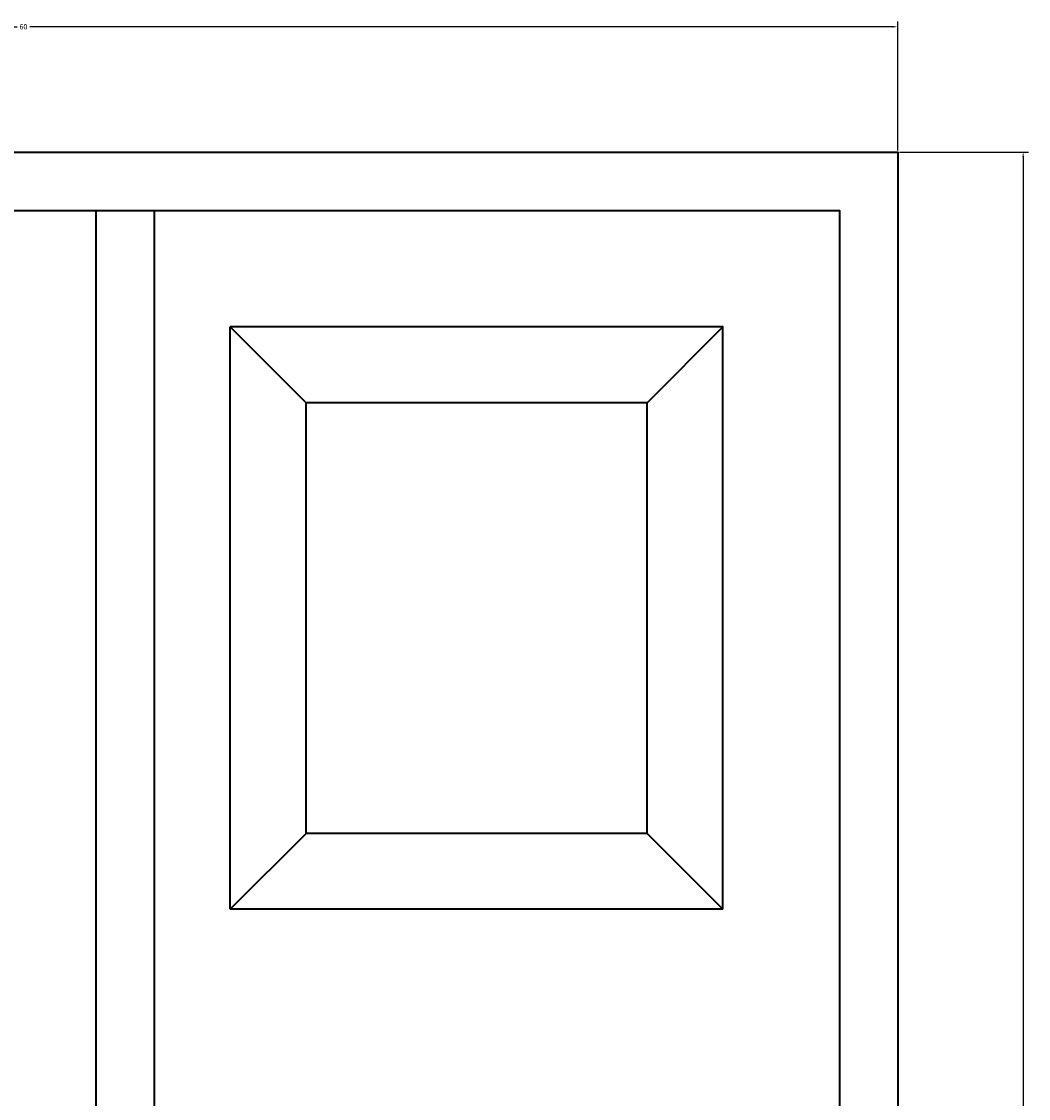
# Model space of a CAD drawing. Units: inches. Extents: x 3137 to 3299, y 1994 to 2089.
# Tile 14 of 14: x 3264 to 3299, y 2052 to 2089. Entities that reach past the tile are written whole.
import ezdxf

# ---------------------------------------------------------------- set-up
doc = ezdxf.new("R2010")
doc.units = ezdxf.units.IN
doc.header["$MEASUREMENT"] = 0
doc.layers.add('A-ANNO-DIMS', color=2, linetype='Continuous', lineweight=18)
doc.layers.add('A-DOOR', color=4, linetype='Continuous', lineweight=35)
doc.styles.get("Standard").update_dxf_attribs({"font": 'arial.ttf'})
doc.dimstyles.get("Standard").update_dxf_attribs({"dimtxt": 0.18, "dimasz": 0.18, "dimexe": 0.18, "dimexo": 0.0625, "dimgap": 0.09, "dimtad": 0, "dimtih": 1, "dimtoh": 1, "dimdec": 4, "dimzin": 0, "dimdsep": 46, "dimtxsty": 'Standard', "dimcen": 0.09, "dimadec": 0, "dimazin": 0, "dimtfac": 1, "dimtdec": 4, "dimtofl": 0, "dimtmove": 0, "dimatfit": 3, "dimfxl": 1, "dimtolj": 1, "dimtzin": 0, "dimarcsym": 0})

# ---------------------------------------------------------------- blocks, each defined once
blk = doc.blocks.new('DOOR-PANEL-RAISED-TOP')
for p, q in [((0, 19.99), (2.6, 17.39)), ((14.3, 17.39), (16.9, 19.99)), ((16.9, 0), (16.9, 19.99)), ((14.3, 2.6), (14.3, 17.39)), ((2.6, 2.6), (0, 0)), ((2.6, 2.6), (14.3, 2.6)), ((14.3, 2.6), (16.9, 0)), ((0, 0), (16.9, 0))]:
    blk.add_line(p, q)
for points in [[(0, 0), (0, 19.99), (16.9, 19.99)], [(2.6, 2.6), (2.6, 17.39), (14.3, 17.39)]]:
    blk.add_lwpolyline(points)
blk = doc.blocks.new('*D74')
at = {"layer": 'A-ANNO-DIMS', "color": 0, "lineweight": -2, "transparency": 16777216}
for p, q in [((3234.504, 2084.238), (3234.504, 2088.661)), ((3294.504, 2084.238), (3294.504, 2088.661)), ((3234.684, 2088.481), (3264.285, 2088.481)), ((3294.324, 2088.481), (3264.723, 2088.481))]:
    blk.add_line(p, q, dxfattribs=at)
at = {"layer": 'A-ANNO-DIMS', "color": 0, "transparency": 16777216}
for points in [[(3234.684, 2088.511), (3234.684, 2088.451), (3234.504, 2088.481)], [(3294.324, 2088.511), (3294.324, 2088.451), (3294.504, 2088.481)]]:
    blk.add_solid(points, dxfattribs=at)
at = {"layer": 'Defpoints', "color": 0, "transparency": 16777216}
for p in [(3294.504, 2088.481), (3234.504, 2084.176), (3294.504, 2084.176)]:
    blk.add_point(p, dxfattribs=at)
at = {"layer": 'A-ANNO-DIMS', "color": 0, "transparency": 16777216, "insert": (3264.504, 2088.481), "char_height": 0.18, "attachment_point": 5}
blk.add_mtext('\\A1;60', dxfattribs=at)
blk = doc.blocks.new('*D75')
at = {"layer": 'A-ANNO-DIMS', "color": 0, "lineweight": -2, "transparency": 16777216}
for p, q in [((3294.566, 2084.176), (3298.989, 2084.176)), ((3298.809, 2083.996), (3298.809, 2042.358)), ((3298.809, 2000.356), (3298.809, 2041.994)), ((3294.566, 2000.176), (3298.989, 2000.176))]:
    blk.add_line(p, q, dxfattribs=at)
at = {"layer": 'A-ANNO-DIMS', "color": 0, "transparency": 16777216}
for points in [[(3298.779, 2083.996), (3298.839, 2083.996), (3298.809, 2084.176)], [(3298.779, 2000.356), (3298.839, 2000.356), (3298.809, 2000.176)]]:
    blk.add_solid(points, dxfattribs=at)
at = {"layer": 'Defpoints', "color": 0, "transparency": 16777216}
for p in [(3294.504, 2084.176), (3298.809, 2084.176), (3294.504, 2000.176)]:
    blk.add_point(p, dxfattribs=at)
at = {"layer": 'A-ANNO-DIMS', "color": 0, "transparency": 16777216, "insert": (3298.809, 2042.176), "char_height": 0.18, "attachment_point": 5}
blk.add_mtext('\\A1;84', dxfattribs=at)

msp = doc.modelspace()

# ---------------------------------------------------------------- linework, layer by layer
at = {"layer": 'A-DOOR'}
for p, q in [((3267.0039, 2028.6759), (3267.0039, 2082.1756)), ((3269.0039, 2028.6759), (3269.0039, 2082.1756))]:
    msp.add_line(p, q, dxfattribs=at)
for points in [[(3234.5039, 2084.1756), (3294.5039, 2084.1756), (3294.5039, 2000.1756), (3234.5039, 2000.1756)], [(3236.5039, 2082.1756), (3292.5039, 2082.1756), (3292.5039, 2002.1756), (3236.5039, 2002.1756)]]:
    msp.add_lwpolyline(points, close=True, dxfattribs=at)

# ---------------------------------------------------------------- block references
at = {"layer": 'A-DOOR', "extrusion": (0, 0, -1), "zscale": -1}
msp.add_blockref('DOOR-PANEL-RAISED-TOP', (-3288.5039, 2058.186), dxfattribs=at)

# ---------------------------------------------------------------- dimensions: what is measured, and where the dimension line sits
at = {"layer": 'A-ANNO-DIMS'}
dim = msp.add_linear_dim(base=(3294.5039, 2088.4806), p1=(3234.5039, 2084.1756), p2=(3294.5039, 2084.1756), dimstyle='Standard', override={"dimdec": 0, "dimlfac": 1, "dimrnd": 0, "dimzin": 0, "dimdsep": 46, "dimlunit": 2}, dxfattribs=at)
dim.commit()
dim.dimension.update_dxf_attribs({"geometry": '*D74', "text_midpoint": (3264.5039, 2088.4806)})
dim = msp.add_linear_dim(base=(3298.8089, 2084.1756), p1=(3294.5039, 2000.1756), p2=(3294.5039, 2084.1756), angle=90, dimstyle='Standard', override={"dimdec": 0, "dimlfac": 1, "dimrnd": 0, "dimzin": 0, "dimdsep": 46, "dimlunit": 2}, dxfattribs=at)
dim.commit()
dim.dimension.update_dxf_attribs({"geometry": '*D75', "text_midpoint": (3298.8089, 2042.1756)})

doc.saveas('drawing.dxf')
